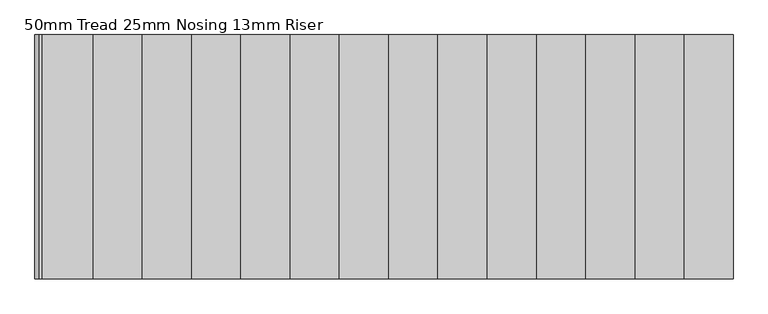
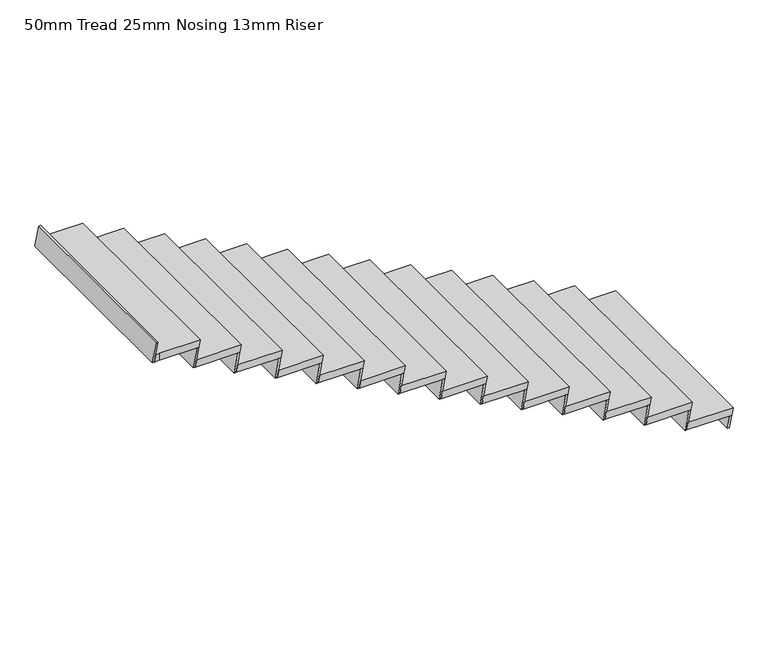
"""IFC4 building model written with IfcOpenShell, lengths in millimetres: stair flight geometry, 50mm Tread 25mm Nosing 13mm Riser."""

from ifc_helpers import new_model, si_unit, origin, place, context, project, spatial, faceted_brep, source, transform, mapped, element, save


def stair_flight_50mm_tread_25mm_nosing_13mm_riser_e3b9914b(model_context):
    return source(origin(), model_context, "Body", "Brep", [
        faceted_brep([(3315.6033064, 215.3469597, 133.3333333), (3306.2283064, 215.3469597, 83.3333333), (3306.2283064, -1149.071626, 83.3333333), (3315.6033064, -1149.071626, 133.3333333), (3615.6033064, -1149.071626, 133.3333333), (3615.6033064, 215.3469597, 133.3333333), (3606.2283064, 215.3469597, 83.3333333), (3606.2283064, -1149.071626, 83.3333333)], [[[0, 1, 2, 3]], [[3, 4, 5, 0]], [[2, 1, 6, 7]], [[4, 3, 2, 7]], [[0, 5, 6, 1]], [[5, 4, 7, 6]]]),
        faceted_brep([(3606.2283064, 215.3469597, 83.3333333), (3590.6033064, 215.3469597, 0.0), (3577.8854778, 215.3469597, 0.0), (3593.5104778, 215.3469597, 83.3333333), (3606.2283064, -1149.071626, 83.3333333), (3593.5104778, -1149.071626, 83.3333333), (3577.8854778, -1149.071626, 0.0), (3590.6033064, -1149.071626, 0.0)], [[[0, 1, 2, 3]], [[4, 5, 6, 7]], [[1, 0, 4, 7]], [[2, 1, 7, 6]], [[3, 2, 6, 5]], [[0, 3, 5, 4]]]),
        faceted_brep([(3331.2283064, 215.3469597, 216.6666667), (3306.2283064, 215.3469597, 83.3333333), (3293.5104778, 215.3469597, 83.3333333), (3318.5104778, 215.3469597, 216.6666667), (3331.2283064, -1149.071626, 216.6666667), (3318.5104778, -1149.071626, 216.6666667), (3293.5104778, -1149.071626, 83.3333333), (3306.2283064, -1149.071626, 83.3333333)], [[[0, 1, 2, 3]], [[4, 5, 6, 7]], [[1, 0, 4, 7]], [[2, 1, 7, 6]], [[3, 2, 6, 5]], [[0, 3, 5, 4]]]),
        faceted_brep([(3040.6033064, -1149.071626, 266.6666667), (3340.6033064, -1149.071626, 266.6666667), (3340.6033064, 215.3469597, 266.6666667), (3040.6033064, 215.3469597, 266.6666667), (3031.2283064, -1149.071626, 216.6666667), (3031.2283064, 215.3469597, 216.6666667), (3331.2283064, 215.3469597, 216.6666667), (3331.2283064, -1149.071626, 216.6666667)], [[[0, 1, 2, 3]], [[4, 5, 6, 7]], [[1, 0, 4, 7]], [[3, 2, 6, 5]], [[3, 5, 4, 0]], [[2, 1, 7, 6]]]),
        faceted_brep([(3056.2283064, 215.3469597, 350.0), (3031.2283064, 215.3469597, 216.6666667), (3018.5104778, 215.3469597, 216.6666667), (3043.5104778, 215.3469597, 350.0), (3056.2283064, -1149.071626, 350.0), (3043.5104778, -1149.071626, 350.0), (3018.5104778, -1149.071626, 216.6666667), (3031.2283064, -1149.071626, 216.6666667)], [[[0, 1, 2, 3]], [[4, 5, 6, 7]], [[1, 0, 4, 7]], [[2, 1, 7, 6]], [[3, 2, 6, 5]], [[0, 3, 5, 4]]]),
        faceted_brep([(2765.6033064, -1149.071626, 400.0), (3065.6033064, -1149.071626, 400.0), (3065.6033064, 215.3469597, 400.0), (2765.6033064, 215.3469597, 400.0), (2756.2283064, -1149.071626, 350.0), (2756.2283064, 215.3469597, 350.0), (3056.2283064, 215.3469597, 350.0), (3056.2283064, -1149.071626, 350.0)], [[[0, 1, 2, 3]], [[4, 5, 6, 7]], [[1, 0, 4, 7]], [[3, 2, 6, 5]], [[3, 5, 4, 0]], [[2, 1, 7, 6]]]),
        faceted_brep([(2781.2283064, 215.3469597, 483.3333333), (2756.2283064, 215.3469597, 350.0), (2743.5104778, 215.3469597, 350.0), (2768.5104778, 215.3469597, 483.3333333), (2781.2283064, -1149.071626, 483.3333333), (2768.5104778, -1149.071626, 483.3333333), (2743.5104778, -1149.071626, 350.0), (2756.2283064, -1149.071626, 350.0)], [[[0, 1, 2, 3]], [[4, 5, 6, 7]], [[1, 0, 4, 7]], [[2, 1, 7, 6]], [[3, 2, 6, 5]], [[0, 3, 5, 4]]]),
        faceted_brep([(2490.6033064, -1149.071626, 533.3333333), (2790.6033064, -1149.071626, 533.3333333), (2790.6033064, 215.3469597, 533.3333333), (2490.6033064, 215.3469597, 533.3333333), (2481.2283064, -1149.071626, 483.3333333), (2481.2283064, 215.3469597, 483.3333333), (2781.2283064, 215.3469597, 483.3333333), (2781.2283064, -1149.071626, 483.3333333)], [[[0, 1, 2, 3]], [[4, 5, 6, 7]], [[1, 0, 4, 7]], [[3, 2, 6, 5]], [[3, 5, 4, 0]], [[2, 1, 7, 6]]]),
        faceted_brep([(2506.2283064, 215.3469597, 616.6666667), (2481.2283064, 215.3469597, 483.3333333), (2468.5104778, 215.3469597, 483.3333333), (2493.5104778, 215.3469597, 616.6666667), (2506.2283064, -1149.071626, 616.6666667), (2493.5104778, -1149.071626, 616.6666667), (2468.5104778, -1149.071626, 483.3333333), (2481.2283064, -1149.071626, 483.3333333)], [[[0, 1, 2, 3]], [[4, 5, 6, 7]], [[1, 0, 4, 7]], [[2, 1, 7, 6]], [[3, 2, 6, 5]], [[0, 3, 5, 4]]]),
        faceted_brep([(2215.6033064, -1149.071626, 666.6666667), (2515.6033064, -1149.071626, 666.6666667), (2515.6033064, 215.3469597, 666.6666667), (2215.6033064, 215.3469597, 666.6666667), (2206.2283064, -1149.071626, 616.6666667), (2206.2283064, 215.3469597, 616.6666667), (2506.2283064, 215.3469597, 616.6666667), (2506.2283064, -1149.071626, 616.6666667)], [[[0, 1, 2, 3]], [[4, 5, 6, 7]], [[1, 0, 4, 7]], [[3, 2, 6, 5]], [[3, 5, 4, 0]], [[2, 1, 7, 6]]]),
        faceted_brep([(2231.2283064, 215.3469597, 750.0), (2206.2283064, 215.3469597, 616.6666667), (2193.5104778, 215.3469597, 616.6666667), (2218.5104778, 215.3469597, 750.0), (2231.2283064, -1149.071626, 750.0), (2218.5104778, -1149.071626, 750.0), (2193.5104778, -1149.071626, 616.6666667), (2206.2283064, -1149.071626, 616.6666667)], [[[0, 1, 2, 3]], [[4, 5, 6, 7]], [[1, 0, 4, 7]], [[2, 1, 7, 6]], [[3, 2, 6, 5]], [[0, 3, 5, 4]]]),
        faceted_brep([(1940.6033064, -1149.071626, 800.0), (2240.6033064, -1149.071626, 800.0), (2240.6033064, 215.3469597, 800.0), (1940.6033064, 215.3469597, 800.0), (1931.2283064, -1149.071626, 750.0), (1931.2283064, 215.3469597, 750.0), (2231.2283064, 215.3469597, 750.0), (2231.2283064, -1149.071626, 750.0)], [[[0, 1, 2, 3]], [[4, 5, 6, 7]], [[1, 0, 4, 7]], [[3, 2, 6, 5]], [[3, 5, 4, 0]], [[2, 1, 7, 6]]]),
        faceted_brep([(1956.2283064, 215.3469597, 883.3333333), (1931.2283064, 215.3469597, 750.0), (1918.5104778, 215.3469597, 750.0), (1943.5104778, 215.3469597, 883.3333333), (1956.2283064, -1149.071626, 883.3333333), (1943.5104778, -1149.071626, 883.3333333), (1918.5104778, -1149.071626, 750.0), (1931.2283064, -1149.071626, 750.0)], [[[0, 1, 2, 3]], [[4, 5, 6, 7]], [[1, 0, 4, 7]], [[2, 1, 7, 6]], [[3, 2, 6, 5]], [[0, 3, 5, 4]]]),
        faceted_brep([(1665.6033064, -1149.071626, 933.3333333), (1965.6033064, -1149.071626, 933.3333333), (1965.6033064, 215.3469597, 933.3333333), (1665.6033064, 215.3469597, 933.3333333), (1656.2283064, -1149.071626, 883.3333333), (1656.2283064, 215.3469597, 883.3333333), (1956.2283064, 215.3469597, 883.3333333), (1956.2283064, -1149.071626, 883.3333333)], [[[0, 1, 2, 3]], [[4, 5, 6, 7]], [[1, 0, 4, 7]], [[3, 2, 6, 5]], [[3, 5, 4, 0]], [[2, 1, 7, 6]]]),
        faceted_brep([(1681.2283064, 215.3469597, 1016.6666667), (1656.2283064, 215.3469597, 883.3333333), (1643.5104778, 215.3469597, 883.3333333), (1668.5104778, 215.3469597, 1016.6666667), (1681.2283064, -1149.071626, 1016.6666667), (1668.5104778, -1149.071626, 1016.6666667), (1643.5104778, -1149.071626, 883.3333333), (1656.2283064, -1149.071626, 883.3333333)], [[[0, 1, 2, 3]], [[4, 5, 6, 7]], [[1, 0, 4, 7]], [[2, 1, 7, 6]], [[3, 2, 6, 5]], [[0, 3, 5, 4]]]),
        faceted_brep([(1390.6033064, -1149.071626, 1066.6666667), (1690.6033064, -1149.071626, 1066.6666667), (1690.6033064, 215.3469597, 1066.6666667), (1390.6033064, 215.3469597, 1066.6666667), (1381.2283064, -1149.071626, 1016.6666667), (1381.2283064, 215.3469597, 1016.6666667), (1681.2283064, 215.3469597, 1016.6666667), (1681.2283064, -1149.071626, 1016.6666667)], [[[0, 1, 2, 3]], [[4, 5, 6, 7]], [[1, 0, 4, 7]], [[3, 2, 6, 5]], [[3, 5, 4, 0]], [[2, 1, 7, 6]]]),
        faceted_brep([(1406.2283064, 215.3469597, 1150.0), (1381.2283064, 215.3469597, 1016.6666667), (1368.5104778, 215.3469597, 1016.6666667), (1393.5104778, 215.3469597, 1150.0), (1406.2283064, -1149.071626, 1150.0), (1393.5104778, -1149.071626, 1150.0), (1368.5104778, -1149.071626, 1016.6666667), (1381.2283064, -1149.071626, 1016.6666667)], [[[0, 1, 2, 3]], [[4, 5, 6, 7]], [[1, 0, 4, 7]], [[2, 1, 7, 6]], [[3, 2, 6, 5]], [[0, 3, 5, 4]]]),
        faceted_brep([(1115.6033064, -1149.071626, 1200.0), (1415.6033064, -1149.071626, 1200.0), (1415.6033064, 215.3469597, 1200.0), (1115.6033064, 215.3469597, 1200.0), (1106.2283064, -1149.071626, 1150.0), (1106.2283064, 215.3469597, 1150.0), (1406.2283064, 215.3469597, 1150.0), (1406.2283064, -1149.071626, 1150.0)], [[[0, 1, 2, 3]], [[4, 5, 6, 7]], [[1, 0, 4, 7]], [[3, 2, 6, 5]], [[3, 5, 4, 0]], [[2, 1, 7, 6]]]),
        faceted_brep([(1131.2283064, 215.3469597, 1283.3333333), (1106.2283064, 215.3469597, 1150.0), (1093.5104778, 215.3469597, 1150.0), (1118.5104778, 215.3469597, 1283.3333333), (1131.2283064, -1149.071626, 1283.3333333), (1118.5104778, -1149.071626, 1283.3333333), (1093.5104778, -1149.071626, 1150.0), (1106.2283064, -1149.071626, 1150.0)], [[[0, 1, 2, 3]], [[4, 5, 6, 7]], [[1, 0, 4, 7]], [[2, 1, 7, 6]], [[3, 2, 6, 5]], [[0, 3, 5, 4]]]),
        faceted_brep([(840.6033064, -1149.071626, 1333.3333333), (1140.6033064, -1149.071626, 1333.3333333), (1140.6033064, 215.3469597, 1333.3333333), (840.6033064, 215.3469597, 1333.3333333), (831.2283064, -1149.071626, 1283.3333333), (831.2283064, 215.3469597, 1283.3333333), (1131.2283064, 215.3469597, 1283.3333333), (1131.2283064, -1149.071626, 1283.3333333)], [[[0, 1, 2, 3]], [[4, 5, 6, 7]], [[1, 0, 4, 7]], [[3, 2, 6, 5]], [[3, 5, 4, 0]], [[2, 1, 7, 6]]]),
        faceted_brep([(856.2283064, 215.3469597, 1416.6666667), (831.2283064, 215.3469597, 1283.3333333), (818.5104778, 215.3469597, 1283.3333333), (843.5104778, 215.3469597, 1416.6666667), (856.2283064, -1149.071626, 1416.6666667), (843.5104778, -1149.071626, 1416.6666667), (818.5104778, -1149.071626, 1283.3333333), (831.2283064, -1149.071626, 1283.3333333)], [[[0, 1, 2, 3]], [[4, 5, 6, 7]], [[1, 0, 4, 7]], [[2, 1, 7, 6]], [[3, 2, 6, 5]], [[0, 3, 5, 4]]]),
        faceted_brep([(565.6033064, -1149.071626, 1466.6666667), (865.6033064, -1149.071626, 1466.6666667), (865.6033064, 215.3469597, 1466.6666667), (565.6033064, 215.3469597, 1466.6666667), (556.2283064, -1149.071626, 1416.6666667), (556.2283064, 215.3469597, 1416.6666667), (856.2283064, 215.3469597, 1416.6666667), (856.2283064, -1149.071626, 1416.6666667)], [[[0, 1, 2, 3]], [[4, 5, 6, 7]], [[1, 0, 4, 7]], [[3, 2, 6, 5]], [[3, 5, 4, 0]], [[2, 1, 7, 6]]]),
        faceted_brep([(581.2283064, 215.3469597, 1550.0), (556.2283064, 215.3469597, 1416.6666667), (543.5104778, 215.3469597, 1416.6666667), (568.5104778, 215.3469597, 1550.0), (581.2283064, -1149.071626, 1550.0), (568.5104778, -1149.071626, 1550.0), (543.5104778, -1149.071626, 1416.6666667), (556.2283064, -1149.071626, 1416.6666667)], [[[0, 1, 2, 3]], [[4, 5, 6, 7]], [[1, 0, 4, 7]], [[2, 1, 7, 6]], [[3, 2, 6, 5]], [[0, 3, 5, 4]]]),
        faceted_brep([(290.6033064, -1149.071626, 1600.0), (590.6033064, -1149.071626, 1600.0), (590.6033064, 215.3469597, 1600.0), (290.6033064, 215.3469597, 1600.0), (281.2283064, -1149.071626, 1550.0), (281.2283064, 215.3469597, 1550.0), (581.2283064, 215.3469597, 1550.0), (581.2283064, -1149.071626, 1550.0)], [[[0, 1, 2, 3]], [[4, 5, 6, 7]], [[1, 0, 4, 7]], [[3, 2, 6, 5]], [[3, 5, 4, 0]], [[2, 1, 7, 6]]]),
        faceted_brep([(306.2283064, 215.3469597, 1683.3333333), (281.2283064, 215.3469597, 1550.0), (268.5104778, 215.3469597, 1550.0), (293.5104778, 215.3469597, 1683.3333333), (306.2283064, -1149.071626, 1683.3333333), (293.5104778, -1149.071626, 1683.3333333), (268.5104778, -1149.071626, 1550.0), (281.2283064, -1149.071626, 1550.0)], [[[0, 1, 2, 3]], [[4, 5, 6, 7]], [[1, 0, 4, 7]], [[2, 1, 7, 6]], [[3, 2, 6, 5]], [[0, 3, 5, 4]]]),
        faceted_brep([(15.6033064, -1149.071626, 1733.3333333), (315.6033064, -1149.071626, 1733.3333333), (315.6033064, 215.3469597, 1733.3333333), (15.6033064, 215.3469597, 1733.3333333), (6.2283064, -1149.071626, 1683.3333333), (6.2283064, 215.3469597, 1683.3333333), (306.2283064, 215.3469597, 1683.3333333), (306.2283064, -1149.071626, 1683.3333333)], [[[0, 1, 2, 3]], [[4, 5, 6, 7]], [[1, 0, 4, 7]], [[3, 2, 6, 5]], [[3, 5, 4, 0]], [[2, 1, 7, 6]]]),
        faceted_brep([(-243.7716936, 215.3469597, 1950.0), (-268.7716936, 215.3469597, 1816.6666667), (-281.4895222, 215.3469597, 1816.6666667), (-256.4895222, 215.3469597, 1950.0), (-243.7716936, -1149.071626, 1950.0), (-256.4895222, -1149.071626, 1950.0), (-281.4895222, -1149.071626, 1816.6666667), (-268.7716936, -1149.071626, 1816.6666667)], [[[0, 1, 2, 3]], [[4, 5, 6, 7]], [[1, 0, 4, 7]], [[2, 1, 7, 6]], [[3, 2, 6, 5]], [[0, 3, 5, 4]]]),
        faceted_brep([(31.2283064, 215.3469597, 1816.6666667), (6.2283064, 215.3469597, 1683.3333333), (-6.4895222, 215.3469597, 1683.3333333), (18.5104778, 215.3469597, 1816.6666667), (31.2283064, -1149.071626, 1816.6666667), (18.5104778, -1149.071626, 1816.6666667), (-6.4895222, -1149.071626, 1683.3333333), (6.2283064, -1149.071626, 1683.3333333)], [[[0, 1, 2, 3]], [[4, 5, 6, 7]], [[1, 0, 4, 7]], [[2, 1, 7, 6]], [[3, 2, 6, 5]], [[0, 3, 5, 4]]]),
        faceted_brep([(-259.3966936, -1149.071626, 1866.6666667), (-234.3966936, -1149.071626, 1866.6666667), (40.6033064, -1149.071626, 1866.6666667), (40.6033064, 215.3469597, 1866.6666667), (-259.3966936, 215.3469597, 1866.6666667), (-268.7716936, -1149.071626, 1816.6666667), (-268.7716936, 215.3469597, 1816.6666667), (31.2283064, 215.3469597, 1816.6666667), (31.2283064, -1149.071626, 1816.6666667), (-234.3966936, -1149.071626, 1816.6666667)], [[[0, 1, 2, 3, 4]], [[5, 6, 7, 8, 9]], [[1, 0, 5, 9]], [[2, 1, 9, 8]], [[4, 3, 7, 6]], [[4, 6, 5, 0]], [[3, 2, 8, 7]]]),
    ])


if __name__ == "__main__":
    model = new_model("IFC4")
    model_context = context("Model", 3, world=origin())
    ifc_project = project(units=[si_unit("LENGTHUNIT", "METRE", prefix="MILLI")], contexts=[model_context])
    site = spatial("IfcSite", under=ifc_project)
    building = spatial("IfcBuilding", under=site)
    placement = place(None, origin())
    stair_flight_50mm_tread_25mm_nosing_13mm_riser_shape = stair_flight_50mm_tread_25mm_nosing_13mm_riser_e3b9914b(model_context)
    element("IfcStairFlight", 1, ObjectType="50mm Tread 25mm Nosing 13mm Riser", at=placement, inside=building, context=model_context, shape_type="MappedRepresentation", body=[
        mapped(stair_flight_50mm_tread_25mm_nosing_13mm_riser_shape, transform((0.0, 0.0, 0.0), x_axis=(1.0, 0.0, 0.0), y_axis=(0.0, 1.0, 0.0), z_axis=(0.0, 0.0, 1.0))),
    ])
    save(model, "model.ifc")
